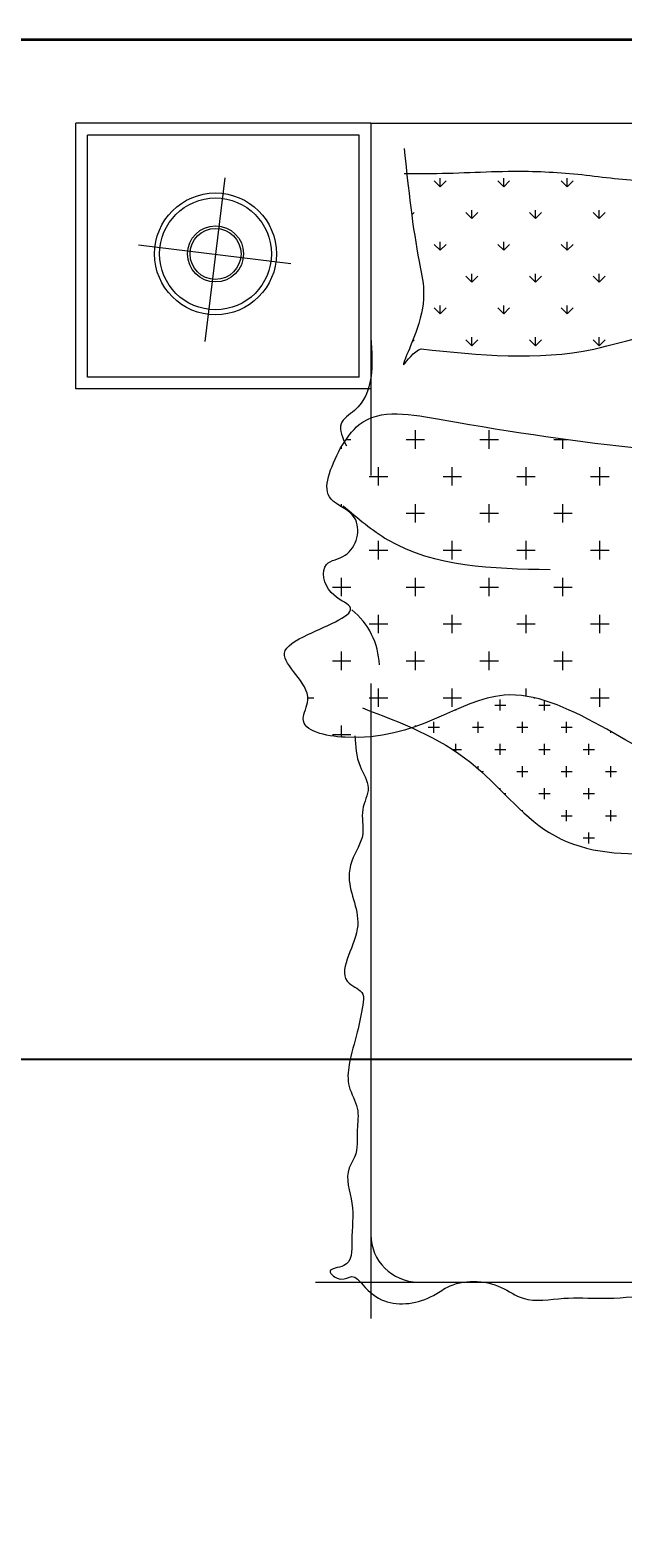
# Model space of a CAD drawing. Units: inches. Extents: x 3731 to 4318, y 1310 to 2388.
# Tile 51 of 57: x 4116 to 4157, y 2229 to 2334. Entities that reach past the tile are written whole.
import ezdxf

# ---------------------------------------------------------------- set-up
doc = ezdxf.new("R2010")
doc.units = ezdxf.units.IN
for name, color, linetype, lineweight in [('A-ANNO-DIMS', 2, 'Continuous', 18), ('A-FURN', 8, 'Continuous', 13), ('A-WALL', 7, 'Continuous', 35)]:
    doc.layers.add(name, color=color, linetype=linetype, lineweight=lineweight)
doc.styles.get("Standard").update_dxf_attribs({"font": 'arial.ttf'})
doc.dimstyles.get("Standard").update_dxf_attribs({"dimtxt": 0.18, "dimasz": 0.18, "dimexe": 0.18, "dimexo": 0.0625, "dimgap": 0.09, "dimtad": 0, "dimtih": 1, "dimtoh": 1, "dimdec": 4, "dimzin": 0, "dimdsep": 46, "dimtxsty": 'Standard', "dimcen": 0.09, "dimadec": 0, "dimazin": 0, "dimtfac": 1, "dimtdec": 4, "dimtofl": 0, "dimtmove": 0, "dimatfit": 3, "dimfxl": 1, "dimtolj": 1, "dimtzin": 0, "dimarcsym": 0})

# ---------------------------------------------------------------- blocks, each defined once
blk = doc.blocks.new('A$C200C7901')
for p, q in [((0, 1.8834), (0, 2.3334)), ((0.5, 2.3334), (0, 2.3334)), ((0.5, 2.3334), (0.5, 1.7369)), ((0.5, 2.3334), (0.5, 1.7369)), ((0.5, 2.3334), (2, 2.3334)), ((0.5701, 1.9635), (0.5733, 1.9666)), ((0.5701, 1.9635), (0.5733, 1.9666)), ((0.5, 1.8834), (0, 1.8834)), ((0.458, 1.7977), (0.466, 1.7977)), ((0.458, 1.7977), (0.466, 1.7977)), ((0.4504, 1.782), (0.4504, 1.7863)), ((0.4504, 1.782), (0.4504, 1.7863)), ((0.4504, 1.6834), (0.4504, 1.6883)), ((0.4504, 1.6834), (0.4504, 1.6883)), ((0.4656, 1.6727), (0.466, 1.6727)), ((0.4656, 1.6727), (0.466, 1.6727)), ((0.5597, 1.6727), (0.591, 1.6727)), ((0.5597, 1.6727), (0.591, 1.6727)), ((0.4504, 1.532), (0.4504, 1.5633)), ((0.4347, 1.5477), (0.466, 1.5477)), ((0.6847, 1.5477), (0.716, 1.5477)), ((0.4347, 1.4227), (0.466, 1.4227)), ((0.5, 1.3845), (0.5, 0.3086)), ((0.3931, 1.3602), (0.4035, 1.3602)), ((0.3931, 1.3602), (0.4035, 1.3602)), ((0.4972, 1.3602), (0.5285, 1.3602)), ((0.4972, 1.3602), (0.5285, 1.3602)), ((0.4504, 1.2936), (0.4504, 1.3133)), ((0.4504, 1.2936), (0.4504, 1.3133)), ((0.4347, 1.2977), (0.466, 1.2977)), ((0.4347, 1.2977), (0.466, 1.2977)), ((0.4061, 0.3703), (2.0386, 0.3703))]:
    blk.add_line(p, q)
at = {"linetype": 'ByBlock'}
for p, q in [((0.02, 1.9034), (0.02, 2.3134)), ((0.48, 2.3134), (0.02, 2.3134)), ((0.48, 1.9034), (0.48, 2.3134)), ((0.2524, 2.2412), (0.2186, 1.9635)), ((0.6171, 2.2259), (0.607, 2.236)), ((0.6171, 2.2259), (0.607, 2.236)), ((0.6171, 2.2259), (0.6171, 2.2402)), ((0.6171, 2.2259), (0.6171, 2.2402)), ((0.6171, 2.2259), (0.6272, 2.236)), ((0.6171, 2.2259), (0.6272, 2.236)), ((0.7249, 2.2259), (0.7148, 2.236)), ((0.7249, 2.2259), (0.7148, 2.236)), ((0.7249, 2.2259), (0.7249, 2.2402)), ((0.7249, 2.2259), (0.7249, 2.2402)), ((0.7249, 2.2259), (0.735, 2.236)), ((0.7249, 2.2259), (0.735, 2.236)), ((0.8326, 2.2259), (0.8225, 2.236)), ((0.8326, 2.2259), (0.8225, 2.236)), ((0.8326, 2.2259), (0.8326, 2.2402)), ((0.8326, 2.2259), (0.8326, 2.2402)), ((0.8326, 2.2259), (0.8427, 2.236)), ((0.8326, 2.2259), (0.8427, 2.236)), ((0.5692, 2.178), (0.5733, 2.1822)), ((0.5692, 2.178), (0.5733, 2.1822)), ((0.671, 2.1721), (0.6609, 2.1822)), ((0.671, 2.1721), (0.6609, 2.1822)), ((0.671, 2.172), (0.671, 2.1863)), ((0.671, 2.172), (0.671, 2.1863)), ((0.671, 2.1721), (0.6811, 2.1822)), ((0.671, 2.1721), (0.6811, 2.1822)), ((0.7787, 2.1721), (0.7686, 2.1822)), ((0.7787, 2.1721), (0.7686, 2.1822)), ((0.7787, 2.172), (0.7787, 2.1863)), ((0.7787, 2.172), (0.7787, 2.1863)), ((0.7787, 2.1721), (0.7889, 2.1822)), ((0.7787, 2.1721), (0.7889, 2.1822)), ((0.8865, 2.1721), (0.8764, 2.1822)), ((0.8865, 2.1721), (0.8764, 2.1822)), ((0.8865, 2.172), (0.8865, 2.1863)), ((0.8865, 2.172), (0.8865, 2.1863)), ((0.8865, 2.1721), (0.8966, 2.1822)), ((0.8865, 2.1721), (0.8966, 2.1822)), ((0.3641, 2.0951), (0.1061, 2.1268)), ((0.6171, 2.1182), (0.607, 2.1283)), ((0.6171, 2.1182), (0.607, 2.1283)), ((0.6171, 2.1182), (0.6171, 2.1325)), ((0.6171, 2.1182), (0.6171, 2.1325)), ((0.6171, 2.1182), (0.6272, 2.1283)), ((0.6171, 2.1182), (0.6272, 2.1283)), ((0.7249, 2.1182), (0.7148, 2.1283)), ((0.7249, 2.1182), (0.7148, 2.1283)), ((0.7249, 2.1182), (0.7249, 2.1325)), ((0.7249, 2.1182), (0.7249, 2.1325)), ((0.7249, 2.1182), (0.735, 2.1283)), ((0.7249, 2.1182), (0.735, 2.1283)), ((0.8326, 2.1182), (0.8225, 2.1283)), ((0.8326, 2.1182), (0.8225, 2.1283)), ((0.8326, 2.1182), (0.8326, 2.1325)), ((0.8326, 2.1182), (0.8326, 2.1325)), ((0.8326, 2.1182), (0.8427, 2.1283)), ((0.8326, 2.1182), (0.8427, 2.1283)), ((0.671, 2.0643), (0.6609, 2.0744)), ((0.671, 2.0643), (0.6609, 2.0744)), ((0.671, 2.0643), (0.671, 2.0786)), ((0.671, 2.0643), (0.671, 2.0786)), ((0.671, 2.0643), (0.6811, 2.0744)), ((0.671, 2.0643), (0.6811, 2.0744)), ((0.7787, 2.0643), (0.7686, 2.0744)), ((0.7787, 2.0643), (0.7686, 2.0744)), ((0.7787, 2.0643), (0.7787, 2.0786)), ((0.7787, 2.0643), (0.7787, 2.0786)), ((0.7787, 2.0643), (0.7889, 2.0744)), ((0.7787, 2.0643), (0.7889, 2.0744)), ((0.8865, 2.0643), (0.8764, 2.0744)), ((0.8865, 2.0643), (0.8764, 2.0744)), ((0.8865, 2.0643), (0.8865, 2.0786)), ((0.8865, 2.0643), (0.8865, 2.0786)), ((0.8865, 2.0643), (0.8966, 2.0744)), ((0.8865, 2.0643), (0.8966, 2.0744)), ((0.6171, 2.0104), (0.607, 2.0205)), ((0.6171, 2.0104), (0.607, 2.0205)), ((0.6171, 2.0104), (0.6171, 2.0247)), ((0.6171, 2.0104), (0.6171, 2.0247)), ((0.6171, 2.0104), (0.6272, 2.0205)), ((0.6171, 2.0104), (0.6272, 2.0205)), ((0.7249, 2.0104), (0.7148, 2.0205)), ((0.7249, 2.0104), (0.7148, 2.0205)), ((0.7249, 2.0104), (0.7249, 2.0247)), ((0.7249, 2.0104), (0.7249, 2.0247)), ((0.7249, 2.0104), (0.735, 2.0205)), ((0.7249, 2.0104), (0.735, 2.0205)), ((0.8326, 2.0104), (0.8225, 2.0205)), ((0.8326, 2.0104), (0.8225, 2.0205)), ((0.8326, 2.0104), (0.8326, 2.0247)), ((0.8326, 2.0104), (0.8326, 2.0247)), ((0.8326, 2.0104), (0.8427, 2.0205)), ((0.8326, 2.0104), (0.8427, 2.0205)), ((0.671, 1.9565), (0.671, 1.9708)), ((0.671, 1.9565), (0.671, 1.9708)), ((0.7787, 1.9565), (0.7787, 1.9708)), ((0.7787, 1.9565), (0.7787, 1.9708)), ((0.8865, 1.9565), (0.8865, 1.9708)), ((0.8865, 1.9565), (0.8865, 1.9708)), ((0.671, 1.9565), (0.6609, 1.9666)), ((0.671, 1.9565), (0.6609, 1.9666)), ((0.671, 1.9565), (0.6811, 1.9666)), ((0.671, 1.9565), (0.6811, 1.9666)), ((0.7787, 1.9565), (0.7686, 1.9666)), ((0.7787, 1.9565), (0.7686, 1.9666)), ((0.7787, 1.9565), (0.7889, 1.9666)), ((0.7787, 1.9565), (0.7889, 1.9666)), ((0.8865, 1.9565), (0.8764, 1.9666)), ((0.8865, 1.9565), (0.8764, 1.9666)), ((0.8865, 1.9565), (0.8966, 1.9666)), ((0.8865, 1.9565), (0.8966, 1.9666)), ((0.48, 1.9034), (0.02, 1.9034)), ((0.5597, 1.7977), (0.591, 1.7977)), ((0.5597, 1.7977), (0.591, 1.7977)), ((0.5754, 1.782), (0.5754, 1.8133)), ((0.5754, 1.782), (0.5754, 1.8133)), ((0.6847, 1.7977), (0.716, 1.7977)), ((0.6847, 1.7977), (0.716, 1.7977)), ((0.7004, 1.782), (0.7004, 1.8133)), ((0.7004, 1.782), (0.7004, 1.8133)), ((0.8097, 1.7977), (0.8331, 1.7977)), ((0.8097, 1.7977), (0.8331, 1.7977)), ((0.8254, 1.782), (0.8254, 1.7987)), ((0.8254, 1.782), (0.8254, 1.7987)), ((0.5129, 1.7195), (0.5129, 1.7508)), ((0.5129, 1.7195), (0.5129, 1.7508)), ((0.6379, 1.7195), (0.6379, 1.7508)), ((0.6379, 1.7195), (0.6379, 1.7508)), ((0.7629, 1.7195), (0.7629, 1.7508)), ((0.7629, 1.7195), (0.7629, 1.7508)), ((0.8879, 1.7195), (0.8879, 1.7508)), ((0.8879, 1.7195), (0.8879, 1.7508)), ((0.4972, 1.7352), (0.5285, 1.7352)), ((0.4972, 1.7352), (0.5285, 1.7352)), ((0.6222, 1.7352), (0.6535, 1.7352)), ((0.6222, 1.7352), (0.6535, 1.7352)), ((0.7472, 1.7352), (0.7785, 1.7352)), ((0.7472, 1.7352), (0.7785, 1.7352)), ((0.8722, 1.7352), (0.9035, 1.7352)), ((0.8722, 1.7352), (0.9035, 1.7352)), ((0.5754, 1.657), (0.5754, 1.6883)), ((0.5754, 1.657), (0.5754, 1.6883)), ((0.7004, 1.657), (0.7004, 1.6883)), ((0.7004, 1.657), (0.7004, 1.6883)), ((0.8254, 1.657), (0.8254, 1.6883)), ((0.8254, 1.657), (0.8254, 1.6883)), ((0.6847, 1.6727), (0.716, 1.6727)), ((0.6847, 1.6727), (0.716, 1.6727)), ((0.8097, 1.6727), (0.841, 1.6727)), ((0.8097, 1.6727), (0.841, 1.6727)), ((0.4972, 1.6102), (0.5285, 1.6102)), ((0.4972, 1.6102), (0.5285, 1.6102)), ((0.5129, 1.5945), (0.5129, 1.6258)), ((0.5129, 1.5945), (0.5129, 1.6258)), ((0.6222, 1.6102), (0.6535, 1.6102)), ((0.6222, 1.6102), (0.6535, 1.6102)), ((0.6379, 1.5945), (0.6379, 1.6258)), ((0.6379, 1.5945), (0.6379, 1.6258)), ((0.7472, 1.6102), (0.7785, 1.6102)), ((0.7472, 1.6102), (0.7785, 1.6102)), ((0.7629, 1.5945), (0.7629, 1.6258)), ((0.7629, 1.5945), (0.7629, 1.6258)), ((0.8722, 1.6102), (0.9035, 1.6102)), ((0.8722, 1.6102), (0.9035, 1.6102)), ((0.8879, 1.5945), (0.8879, 1.6258)), ((0.8879, 1.5945), (0.8879, 1.6258)), ((0.4504, 1.532), (0.4504, 1.5633)), ((0.5754, 1.532), (0.5754, 1.5633)), ((0.5754, 1.532), (0.5754, 1.5633)), ((0.7004, 1.532), (0.7004, 1.5633)), ((0.7004, 1.532), (0.7004, 1.5633)), ((0.8254, 1.532), (0.8254, 1.5633)), ((0.8254, 1.532), (0.8254, 1.5633)), ((0.4347, 1.5477), (0.466, 1.5477)), ((0.5597, 1.5477), (0.591, 1.5477)), ((0.5597, 1.5477), (0.591, 1.5477)), ((0.6847, 1.5477), (0.716, 1.5477)), ((0.8097, 1.5477), (0.841, 1.5477)), ((0.8097, 1.5477), (0.841, 1.5477)), ((0.4972, 1.4852), (0.5285, 1.4852)), ((0.4972, 1.4852), (0.5285, 1.4852)), ((0.5129, 1.4695), (0.5129, 1.5008)), ((0.5129, 1.4695), (0.5129, 1.5008)), ((0.6222, 1.4852), (0.6535, 1.4852)), ((0.6222, 1.4852), (0.6535, 1.4852)), ((0.6379, 1.4695), (0.6379, 1.5008)), ((0.6379, 1.4695), (0.6379, 1.5008)), ((0.7472, 1.4852), (0.7785, 1.4852)), ((0.7472, 1.4852), (0.7785, 1.4852)), ((0.7629, 1.4695), (0.7629, 1.5008)), ((0.7629, 1.4695), (0.7629, 1.5008)), ((0.8722, 1.4852), (0.9035, 1.4852)), ((0.8722, 1.4852), (0.9035, 1.4852)), ((0.8879, 1.4695), (0.8879, 1.5008)), ((0.8879, 1.4695), (0.8879, 1.5008)), ((0.4504, 1.407), (0.4504, 1.4383)), ((0.4504, 1.407), (0.4504, 1.4383)), ((0.5754, 1.407), (0.5754, 1.4383)), ((0.5754, 1.407), (0.5754, 1.4383)), ((0.7004, 1.407), (0.7004, 1.4383)), ((0.7004, 1.407), (0.7004, 1.4383)), ((0.8254, 1.407), (0.8254, 1.4383)), ((0.8254, 1.407), (0.8254, 1.4383)), ((0.4347, 1.4227), (0.466, 1.4227)), ((0.5597, 1.4227), (0.591, 1.4227)), ((0.5597, 1.4227), (0.591, 1.4227)), ((0.6847, 1.4227), (0.716, 1.4227)), ((0.6847, 1.4227), (0.716, 1.4227)), ((0.8097, 1.4227), (0.841, 1.4227)), ((0.8097, 1.4227), (0.841, 1.4227)), ((0.5129, 1.3445), (0.5129, 1.3758)), ((0.5129, 1.3445), (0.5129, 1.3758)), ((0.6222, 1.3602), (0.6535, 1.3602)), ((0.6222, 1.3602), (0.6535, 1.3602)), ((0.6379, 1.3445), (0.6379, 1.3758)), ((0.6379, 1.3445), (0.6379, 1.3758)), ((0.7191, 1.3383), (0.7191, 1.357)), ((0.7191, 1.3383), (0.7191, 1.357)), ((0.7629, 1.3627), (0.7629, 1.3758)), ((0.7629, 1.3627), (0.7629, 1.3758)), ((0.7762, 1.3602), (0.7785, 1.3602)), ((0.7762, 1.3602), (0.7785, 1.3602)), ((0.7941, 1.3383), (0.7941, 1.3554)), ((0.7941, 1.3383), (0.7941, 1.3554)), ((0.8722, 1.3602), (0.9035, 1.3602)), ((0.8722, 1.3602), (0.9035, 1.3602)), ((0.8879, 1.3445), (0.8879, 1.3758)), ((0.8879, 1.3445), (0.8879, 1.3758)), ((0.6441, 1.3383), (0.6441, 1.3399)), ((0.6441, 1.3383), (0.6441, 1.3399)), ((0.7097, 1.3477), (0.7285, 1.3477)), ((0.7097, 1.3477), (0.7285, 1.3477)), ((0.7847, 1.3477), (0.8035, 1.3477)), ((0.7847, 1.3477), (0.8035, 1.3477)), ((0.5754, 1.3115), (0.5754, 1.3133)), ((0.5754, 1.3115), (0.5754, 1.3133)), ((0.5972, 1.3102), (0.616, 1.3102)), ((0.5972, 1.3102), (0.616, 1.3102)), ((0.6066, 1.3008), (0.6066, 1.3195)), ((0.6066, 1.3008), (0.6066, 1.3195)), ((0.6722, 1.3102), (0.691, 1.3102)), ((0.6722, 1.3102), (0.691, 1.3102)), ((0.6816, 1.3008), (0.6816, 1.3195)), ((0.6816, 1.3008), (0.6816, 1.3195)), ((0.7472, 1.3102), (0.766, 1.3102)), ((0.7472, 1.3102), (0.766, 1.3102)), ((0.7566, 1.3008), (0.7566, 1.3195)), ((0.7566, 1.3008), (0.7566, 1.3195)), ((0.8222, 1.3102), (0.841, 1.3102)), ((0.8222, 1.3102), (0.841, 1.3102)), ((0.8316, 1.3008), (0.8316, 1.3195)), ((0.8316, 1.3008), (0.8316, 1.3195)), ((0.9066, 1.3008), (0.9066, 1.3028)), ((0.9066, 1.3008), (0.9066, 1.3028)), ((0.6441, 1.2686), (0.6441, 1.282)), ((0.6441, 1.2686), (0.6441, 1.282)), ((0.7191, 1.2633), (0.7191, 1.282)), ((0.7191, 1.2633), (0.7191, 1.282)), ((0.7941, 1.2633), (0.7941, 1.282)), ((0.7941, 1.2633), (0.7941, 1.282)), ((0.8691, 1.2633), (0.8691, 1.282)), ((0.8691, 1.2633), (0.8691, 1.282)), ((0.6379, 1.2727), (0.6535, 1.2727)), ((0.6379, 1.2727), (0.6535, 1.2727)), ((0.7097, 1.2727), (0.7285, 1.2727)), ((0.7097, 1.2727), (0.7285, 1.2727)), ((0.7847, 1.2727), (0.8035, 1.2727)), ((0.7847, 1.2727), (0.8035, 1.2727)), ((0.8597, 1.2727), (0.8785, 1.2727)), ((0.8597, 1.2727), (0.8785, 1.2727)), ((0.6816, 1.2398), (0.6816, 1.2445)), ((0.6816, 1.2398), (0.6816, 1.2445)), ((0.6868, 1.2352), (0.691, 1.2352)), ((0.6868, 1.2352), (0.691, 1.2352)), ((0.7472, 1.2352), (0.766, 1.2352)), ((0.7472, 1.2352), (0.766, 1.2352)), ((0.7566, 1.2258), (0.7566, 1.2445)), ((0.7566, 1.2258), (0.7566, 1.2445)), ((0.8222, 1.2352), (0.841, 1.2352)), ((0.8222, 1.2352), (0.841, 1.2352)), ((0.8316, 1.2258), (0.8316, 1.2445)), ((0.8316, 1.2258), (0.8316, 1.2445)), ((0.8972, 1.2352), (0.916, 1.2352)), ((0.8972, 1.2352), (0.916, 1.2352)), ((0.9066, 1.2258), (0.9066, 1.2445)), ((0.9066, 1.2258), (0.9066, 1.2445)), ((0.7191, 1.2041), (0.7191, 1.207)), ((0.7191, 1.2041), (0.7191, 1.207)), ((0.7941, 1.1883), (0.7941, 1.207)), ((0.7941, 1.1883), (0.7941, 1.207)), ((0.8691, 1.1883), (0.8691, 1.207)), ((0.8691, 1.1883), (0.8691, 1.207)), ((0.7255, 1.1977), (0.7285, 1.1977)), ((0.7255, 1.1977), (0.7285, 1.1977)), ((0.7847, 1.1977), (0.8035, 1.1977)), ((0.7847, 1.1977), (0.8035, 1.1977)), ((0.8597, 1.1977), (0.8785, 1.1977)), ((0.8597, 1.1977), (0.8785, 1.1977)), ((0.7566, 1.1674), (0.7566, 1.1695)), ((0.7566, 1.1674), (0.7566, 1.1695)), ((0.7646, 1.1602), (0.766, 1.1602)), ((0.7646, 1.1602), (0.766, 1.1602)), ((0.8222, 1.1602), (0.841, 1.1602)), ((0.8222, 1.1602), (0.841, 1.1602)), ((0.8316, 1.1508), (0.8316, 1.1695)), ((0.8316, 1.1508), (0.8316, 1.1695)), ((0.8972, 1.1602), (0.916, 1.1602)), ((0.8972, 1.1602), (0.916, 1.1602)), ((0.9066, 1.1508), (0.9066, 1.1695)), ((0.9066, 1.1508), (0.9066, 1.1695)), ((0.8691, 1.1133), (0.8691, 1.132)), ((0.8691, 1.1133), (0.8691, 1.132)), ((0.8597, 1.1227), (0.8785, 1.1227)), ((0.8597, 1.1227), (0.8785, 1.1227))]:
    blk.add_line(p, q, dxfattribs=at)
for radius in [0.1032, 0.0947, 0.0475, 0.0432]:
    blk.add_circle((0.2367, 2.1121), radius, dxfattribs=at)
blk.add_arc((0.3888, 1.4113), 0.1256, 1.9962, 51.1646, dxfattribs=at)
for centre, radius, start, end in [((0.3888, 1.4113), 0.1256, 1.9962, 51.1646), ((0.58, 0.4503), 0.08, 180, 270)]:
    blk.add_arc(centre, radius, start, end)
for points, knots in [([(0.5562, 2.2908), (0.5634, 2.223), (0.5751, 2.1147), (0.6005, 2.0213), (0.5392, 1.8966), (0.5726, 1.9486), (0.5854, 1.951)], [0, 0, 0, 0, 193.119101, 308.278592, 371.468985, 410.593498, 410.593498, 410.593498, 410.593498]), ([(0.5854, 1.951), (0.6835, 1.9407), (0.8425, 1.9242), (1.0374, 2.0054), (1.1564, 1.9255), (1.2274, 1.9841), (1.2052, 2.0751), (1.1815, 2.152), (1.2176, 2.2368), (1.0992, 2.2731), (1.0008, 2.2255), (0.8698, 2.246), (0.7481, 2.2548), (0.6426, 2.2473), (0.5746, 2.2478), (0.5562, 2.2479)], [0, 0, 0, 0, 292.165466, 473.33038, 601.631673, 630.723769, 727.138505, 836.819956, 887.958136, 954.42438, 1118.989809, 1227.016542, 1338.750986, 1487.447361, 1542.751028, 1542.751028, 1542.751028, 1542.751028]), ([(0.4485, 1.7835), (0.4321, 1.7496), (0.4062, 1.6964), (0.49, 1.6713), (0.4719, 1.5969), (0.4123, 1.592), (0.4233, 1.5337), (0.4954, 1.5086), (0.4012, 1.4738), (0.3253, 1.4306), (0.4113, 1.3764), (0.3688, 1.3065), (0.5579, 1.2663), (0.741, 1.4533), (1.1127, 1.1109), (1.4811, 1.2478), (1.7885, 1.3492), (2.0357, 1.1637), (2.0748, 1.2974), (2.0876, 1.349), (2.0192, 1.3805), (2.0564, 1.4298), (2.0588, 1.4846), (1.9759, 1.5349), (2.1004, 1.5845), (2.0397, 1.6519), (1.971, 1.7053), (2.1104, 1.8981), (1.5946, 1.7967), (1.2448, 1.7472), (0.8129, 1.7935), (0.4953, 1.8548), (0.4582, 1.7983), (0.4485, 1.7835)], [0, 0, 0, 0, 88.420092, 139.08588, 204.302936, 239.695496, 287.801042, 327.365471, 412.960499, 463.626286, 552.059846, 584.668336, 662.614915, 940.993281, 1309.926334, 1844.022653, 1996.276242, 2316.43048, 2341.441004, 2404.707416, 2449.463774, 2514.680778, 2538.40571, 2613.031547, 2697.13096, 2760.903931, 2822.692699, 2945.47, 3215.060018, 3725.584917, 4361.974444, 4504.671998, 4555.32777, 4555.32777, 4555.32777, 4555.32777]), ([(0.4856, 1.3429), (0.5504, 1.3182), (0.6715, 1.2721), (0.8374, 1.0498), (1.1164, 1.1183), (1.3878, 1.1816), (1.5888, 1.1102), (1.8403, 1.1127), (1.9415, 1.2178), (2.0032, 1.2819)], [0, 0, 0, 0, 205.411753, 383.654933, 772.067458, 921.644661, 1226.793228, 1388.983508, 1642.292305, 1642.292305, 1642.292305, 1642.292305])]:
    blk.add_open_spline(points, degree=3, knots=knots)
for points, knots in [([(0.5, 1.9703), (0.5029, 1.9235), (0.5066, 1.8648), (0.4398, 1.8252), (0.452, 1.8005), (0.4585, 1.7872)], [0, 0, 0, 0, 126.315232, 158.854004, 196.789047, 196.789047, 196.789047, 196.789047]), ([(0.5, 1.9703), (0.5029, 1.9235), (0.5066, 1.8648), (0.4398, 1.8252), (0.452, 1.8005), (0.4585, 1.7872)], [0, 0, 0, 0, 126.315232, 158.854004, 196.789047, 196.789047, 196.789047, 196.789047]), ([(0.4532, 1.6853), (0.4776, 1.6644), (0.574, 1.582), (0.7055, 1.5794), (0.8037, 1.5774)], [0, 0, 0, 0, 94.920667, 374.457292, 374.457292, 374.457292, 374.457292]), ([(0.4532, 1.6853), (0.4776, 1.6644), (0.574, 1.582), (0.7055, 1.5794), (0.8037, 1.5774)], [0, 0, 0, 0, 94.920667, 374.457292, 374.457292, 374.457292, 374.457292]), ([(0.473, 1.2954), (0.4739, 1.2781), (0.4755, 1.2477), (0.5032, 1.2084), (0.4801, 1.1701), (0.4928, 1.1255), (0.4674, 1.0912), (0.4579, 1.0351), (0.501, 0.9724), (0.4311, 0.8832), (0.4902, 0.8637), (0.4843, 0.8288), (0.4774, 0.7906), (0.4625, 0.7457), (0.459, 0.6999), (0.4816, 0.6664), (0.4748, 0.625), (0.4791, 0.5889), (0.4533, 0.5528), (0.4738, 0.5004), (0.4658, 0.4502), (0.4696, 0.3946), (0.4189, 0.3935), (0.4493, 0.3684), (0.4694, 0.3857), (0.4922, 0.3576), (0.5297, 0.3262), (0.5917, 0.3353), (0.6454, 0.3754), (0.7083, 0.3741), (0.7643, 0.3328), (0.826, 0.346), (0.925, 0.3388), (1.0353, 0.3593), (1.1561, 0.3744), (1.2477, 0.3154), (1.3302, 0.3474), (1.4086, 0.3512), (1.5217, 0.3878), (1.6362, 0.3176), (1.7682, 0.3285), (1.8402, 0.3019), (1.9071, 0.3529), (1.9647, 0.3412), (2.0795, 0.2948), (2.0472, 0.3498), (2.0343, 0.3772), (2.0435, 0.43), (2.0109, 0.5782), (2.0746, 0.4643), (2.0805, 0.584), (2.0084, 0.5979), (2.0343, 0.6846), (2.0344, 0.746), (2.0293, 0.8096), (2.0489, 0.8545), (2.0652, 0.9218), (1.9842, 0.9297), (2.0007, 1.0162), (2.0367, 1.0585), (2.0367, 1.1102), (2.0457, 1.1647), (2.0226, 1.2084), (2.0234, 1.2306), (2.0236, 1.2352)], [0, 0, 0, 0, 51.660678, 90.967412, 128.902454, 170.303599, 219.852997, 247.834962, 336.321557, 429.35469, 458.821847, 477.222321, 524.135809, 581.038434, 617.839381, 657.146115, 693.947125, 740.178081, 760.753248, 820.731705, 885.133458, 928.777044, 953.563729, 976.574207, 995.553042, 1018.563482, 1064.584401, 1147.951297, 1174.787598, 1266.851571, 1308.018447, 1377.066427, 1441.511314, 1608.245014, 1714.11869, 1792.771707, 1913.247991, 1954.931389, 2029.864445, 2259.189419, 2305.221512, 2429.507982, 2456.344283, 2543.92595, 2627.925037, 2662.96218, 2687.736879, 2719.937755, 2839.540991, 2875.47895, 2953.681041, 2993.270313, 3066.872333, 3154.395764, 3200.397042, 3248.426375, 3312.828127, 3347.881398, 3444.484026, 3481.577522, 3518.665244, 3592.267265, 3644.719162, 3658.519501, 3658.519501, 3658.519501, 3658.519501])]:
    blk.add_open_spline(points, degree=3, knots=knots, dxfattribs=at)
blk = doc.blocks.new('*D37')
at = {"layer": 'A-ANNO-DIMS', "color": 0, "lineweight": -2, "transparency": 16777216}
for p, q in [((4239.27, 2338.38), (4318.34, 2338.38)), ((4318.16, 2338.2), (4318.16, 2300.56)), ((4318.16, 2262.56), (4318.16, 2300.2)), ((4103.27, 2262.38), (4318.34, 2262.38))]:
    blk.add_line(p, q, dxfattribs=at)
at = {"layer": 'A-ANNO-DIMS', "color": 0, "transparency": 16777216}
for points in [[(4318.13, 2338.2), (4318.19, 2338.2), (4318.16, 2338.38)], [(4318.13, 2262.56), (4318.19, 2262.56), (4318.16, 2262.38)]]:
    blk.add_solid(points, dxfattribs=at)
at = {"layer": 'Defpoints', "color": 0, "transparency": 16777216}
for p in [(4239.21, 2338.38), (4318.16, 2338.38), (4103.21, 2262.38)]:
    blk.add_point(p, dxfattribs=at)
at = {"layer": 'A-ANNO-DIMS', "color": 0, "transparency": 16777216, "insert": (4318.16, 2300.38), "char_height": 0.18, "attachment_point": 5}
blk.add_mtext('\\A1;76', dxfattribs=at)
blk = doc.blocks.new('*D38')
at = {"layer": 'A-ANNO-DIMS', "color": 0, "lineweight": -2, "transparency": 16777216}
for p, q in [((4103.27, 2262.38), (4318.34, 2262.38)), ((4318.16, 2262.2), (4318.16, 2103.06)), ((4318.16, 1943.56), (4318.16, 2102.7)), ((4234.27, 1943.38), (4318.34, 1943.38))]:
    blk.add_line(p, q, dxfattribs=at)
at = {"layer": 'A-ANNO-DIMS', "color": 0, "transparency": 16777216}
for points in [[(4318.13, 2262.2), (4318.19, 2262.2), (4318.16, 2262.38)], [(4318.13, 1943.56), (4318.19, 1943.56), (4318.16, 1943.38)]]:
    blk.add_solid(points, dxfattribs=at)
at = {"layer": 'Defpoints', "color": 0, "transparency": 16777216}
for p in [(4103.21, 2262.38), (4318.16, 2262.38), (4234.21, 1943.38)]:
    blk.add_point(p, dxfattribs=at)
at = {"layer": 'A-ANNO-DIMS', "color": 0, "transparency": 16777216, "insert": (4318.16, 2102.88), "char_height": 0.18, "attachment_point": 5}
blk.add_mtext('\\A1;319', dxfattribs=at)

msp = doc.modelspace()

# ---------------------------------------------------------------- linework, layer by layer
at = {"layer": 'A-WALL'}
msp.add_line((4108.21, 2333.38), (4234.21, 2333.38), dxfattribs=at)

# ---------------------------------------------------------------- block references
at = {"layer": 'A-FURN', "xscale": 41.1071563136412, "yscale": 41.1071563136412, "zscale": 41.1071563136412}
msp.add_blockref('A$C200C7901', (4119, 2231.63), dxfattribs=at)

# ---------------------------------------------------------------- dimensions: what is measured, and where the dimension line sits
at = {"layer": 'A-ANNO-DIMS'}
for base, p1, p2, picture, middle in [((4318.16, 2338.38), (4103.21, 2262.38), (4239.21, 2338.38), '*D37', (4318.16, 2300.38)), ((4318.16, 2262.38), (4234.21, 1943.38), (4103.21, 2262.38), '*D38', (4318.16, 2102.88))]:
    dim = msp.add_linear_dim(base=base, p1=p1, p2=p2, angle=90, dimstyle='Standard', override={"dimdec": 0, "dimlfac": 1, "dimrnd": 0, "dimzin": 0, "dimdsep": 46, "dimlunit": 2}, dxfattribs=at)
    dim.commit()
    dim.dimension.update_dxf_attribs({"geometry": picture, "text_midpoint": middle})

doc.saveas('drawing.dxf')
